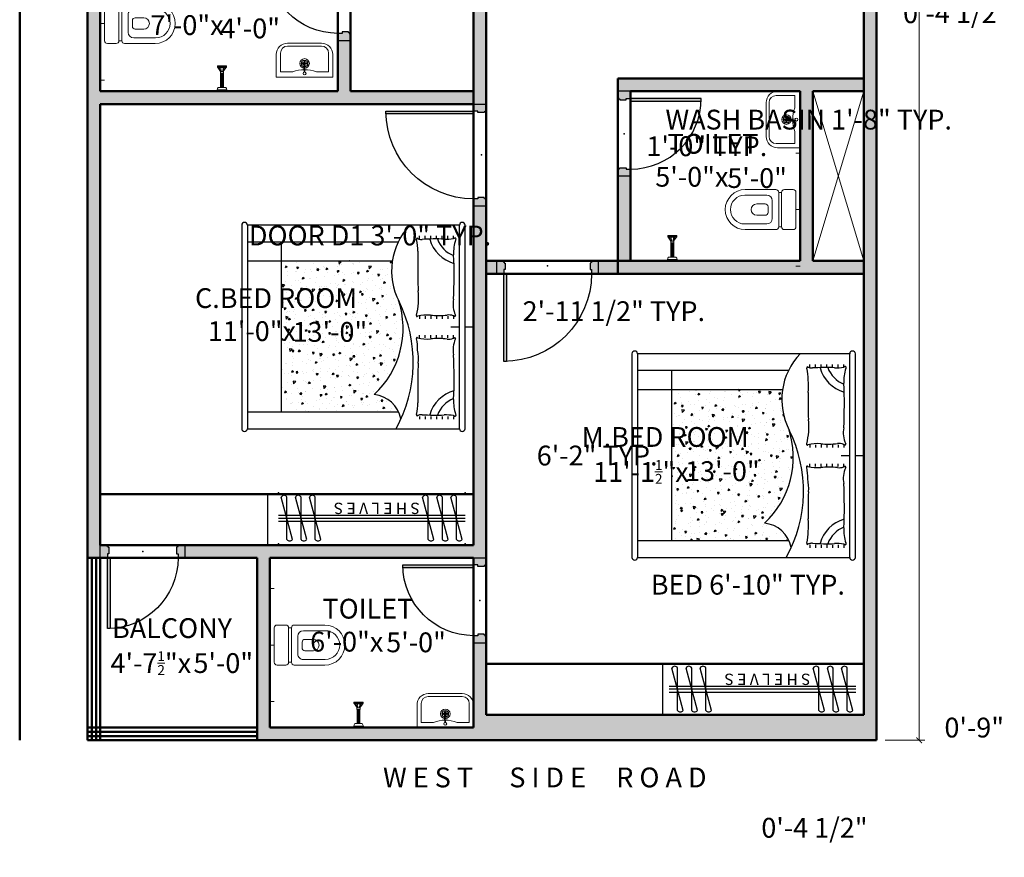
# Model space of a CAD drawing. Units: inches. Extents: x 4508 to 5907, y 877 to 1592.
# Tile 1 of 20: x 4571 to 4919, y 885 to 1182. Entities that reach past the tile are written whole.
import ezdxf

# ---------------------------------------------------------------- set-up
doc = ezdxf.new("R2010")
doc.units = ezdxf.units.IN
doc.layers.get('DEFPOINTS').update_dxf_attribs({"color": 8})
for name, color, linetype, lineweight in [('A-ANNO-DIMS', 2, 'Continuous', 18), ('A-ANNO-TEXT', 7, 'Continuous', 25), ('A-DOOR', 4, 'Continuous', 25), ('A-FLOR-CASE', 30, 'Continuous', 25), ('A-FLOR-FIXT', 8, 'Continuous', 18), ('A-FLOR-SHFT', 8, 'Continuous', 18), ('A-FURN', 24, 'Continuous', 18), ('A-WALL', 7, 'Continuous', 50), ('A-WALL-PATT', 8, 'Continuous', 13)]:
    doc.layers.add(name, color=color, linetype=linetype, lineweight=lineweight)
doc.layers.add('doors & windows', color=30, linetype='Continuous')
doc.layers.add('furniture', color=24, linetype='Continuous')
doc.styles.get("Standard").update_dxf_attribs({"font": 'arial.ttf'})
doc.dimstyles.new('details', dxfattribs={"dimtxt": 5, "dimasz": 2, "dimexe": 2, "dimexo": 3, "dimgap": 1, "dimtad": 0, "dimdec": 1, "dimzin": 0, "dimdsep": 46, "dimlunit": 4, "dimtxsty": 'Standard', "dimblk": 'ARCHTICK', "dimcen": 3, "dimclrd": 256, "dimclre": 256, "dimclrt": 256, "dimadec": 0, "dimazin": 0, "dimtfac": 0.5, "dimtdec": 1, "dimtofl": 0, "dimtmove": 0, "dimatfit": 3, "dimldrblk": 'CLOSEDBLANK', "dimfxl": 2, "dimtolj": 1, "dimtzin": 0, "dimlwd": -1, "dimlwe": -1, "dimarcsym": 0})
doc.dimstyles.new('text', dxfattribs={"dimtxt": 7, "dimasz": 0, "dimexe": 3, "dimexo": 3, "dimgap": 0, "dimtad": 1, "dimtih": 1, "dimtoh": 1, "dimzin": 3, "dimdsep": 46, "dimlunit": 4, "dimtxsty": 'Standard', "dimblk": 'CLOSEDBLANK', "dimcen": 3, "dimse1": 1, "dimse2": 1, "dimsd1": 1, "dimsd2": 1, "dimclrd": 256, "dimclre": 256, "dimclrt": 256, "dimadec": 0, "dimazin": 0, "dimtfac": 0.5, "dimtofl": 0, "dimtmove": 0, "dimatfit": 3, "dimfxl": 3, "dimtolj": 1, "dimtzin": 0, "dimlwd": -1, "dimlwe": -1, "dimarcsym": 0})

# ---------------------------------------------------------------- blocks, each defined once
blk = doc.blocks.new('*D34')
at = {"layer": 'DEFPOINTS', "color": 0, "transparency": 16777216}
for p in [(4683.74, 1178.32), (4683.74, 1175.99), (4599.74, 1170.14)]:
    blk.add_point(p, dxfattribs=at)
at = {"layer": 'A-ANNO-DIMS', "color": 0, "transparency": 16777216, "insert": (4630.42, 1185.46), "char_height": 7, "attachment_point": 5}
blk.add_mtext('\\A1;       TOILET\\P7\'-0"x', dxfattribs=at)
blk = doc.blocks.new('_ClosedBlank')
at = {"color": 0, "lineweight": -2}
for p, q in [((-1, 0.17), (0, 0)), ((-1, 0.17), (-1, -0.17)), ((0, 0), (-1, -0.17))]:
    blk.add_line(p, q, dxfattribs=at)
blk = doc.blocks.new('*D35')
at = {"layer": 'DEFPOINTS', "color": 0, "transparency": 16777216}
for p in [(4647.76, 1204.2), (4647.07, 1156.2), (4652.75, 1156.2)]:
    blk.add_point(p, dxfattribs=at)
at = {"layer": 'A-ANNO-DIMS', "color": 0, "transparency": 16777216, "insert": (4652.75, 1178.45), "char_height": 7, "attachment_point": 5}
blk.add_mtext('\\A1;4\'-0"', dxfattribs=at)
blk = doc.blocks.new('D2')
at = {"layer": 'doors & windows'}
h = blk.add_hatch(dxfattribs=at)
h.set_pattern_fill('DOTS', color=256, scale=2, angle=180, style=0)
h.set_pattern_definition([(180, (0, -4), (-0.0625, -0.125), [0, -0.125])])
h.paths.add_polyline_path([(2.5, 0), (3.5, 0), (3.5, 24.98, 0.010003), (2.5, 25)])
h = blk.add_hatch(dxfattribs=at)
h.set_pattern_fill('DOTS', color=256, scale=2, angle=180, style=0)
h.set_pattern_definition([(180, (0, 0), (-0.0625, -0.125), [0, -0.125])])
edge = h.paths.add_edge_path()
edge.add_line((27.5, 0), (27.5, -1.5))
edge.add_line((27.5, -1.5), (27, -1.5))
edge.add_line((27, -1.5), (27, -3.75))
edge.add_line((27, -3.75), (27.25, -3.75))
edge.add_arc((27.76, -3.74), 0.509, 181.0059, 268.9941)
edge.add_line((27.75, -4.25), (27.75, -4.5))
edge.add_line((27.75, -4.5), (30, -4.5))
edge.add_line((30, -4.5), (30, 0))
edge.add_line((30, 0), (27.5, 0))
edge = h.paths.add_edge_path()
edge.add_line((2.5, -1.5), (2.5, 0))
edge.add_line((2.5, 0), (0, 0))
edge.add_line((0, 0), (0, -4.5))
edge.add_line((0, -4.5), (2.25, -4.5))
edge.add_line((2.25, -4.5), (2.25, -4.25))
edge.add_arc((2.24, -3.74), 0.509, 271.0059, 358.9941)
edge.add_line((2.75, -3.75), (3, -3.75))
edge.add_line((3, -3.75), (3, -1.5))
edge.add_line((3, -1.5), (2.5, -1.5))
for p, q in [((0, 0), (0, -4.5)), ((30, 0), (30, -4.5))]:
    blk.add_line(p, q)
blk.add_lwpolyline([(3.5, 0), (3.5, 25), (2.5, 25), (2.5, 0)], close=True, dxfattribs=at)
for points in [[(3, -3.75), (3, -1.5), (2.5, -1.5), (2.5, 0), (0, 0)], [(27, -3.75), (27, -1.5), (27.5, -1.5), (27.5, 0), (30, 0)], [(0, -4.5), (2.25, -4.5)], [(30, -4.5), (27.75, -4.5)]]:
    blk.add_lwpolyline(points, dxfattribs=at)
for points in [[(2.25, -4.5), (2.25, -4.25, 0.403966), (2.75, -3.75), (3, -3.75)], [(27.75, -4.5), (27.75, -4.25, -0.403966), (27.25, -3.75), (27, -3.75)]]:
    blk.add_lwpolyline(points, format="xyb", dxfattribs=at)
at = {"layer": 'doors & windows', "ltscale": 6}
blk.add_arc((2.5, 0), 25, 0, 90, dxfattribs=at)
at = {"layer": 'doors & windows'}
blk.add_point((15, -2.25), dxfattribs=at)
blk = doc.blocks.new('commode')
for p, q in [((-7.09, 19.41), (-7.09, 8.61)), ((-5.09, 11.81), (-5.09, 19.57)), ((5.09, 11.81), (5.09, 19.57)), ((7.09, 19.41), (7.09, 8.61)), ((-2, 12.37), (-2, 15.37)), ((2, 12.37), (2, 15.37)), ((-1, 11.37), (1, 11.37)), ((-6.09, 7.61), (6.09, 7.61)), ((-6.09, 6.61), (-6.09, 7.61)), ((-3.15, 9.87), (3.15, 9.87)), ((6.09, 7.61), (6.09, 6.61)), ((-7.09, 2.5), (-7.09, 5.61)), ((-6.09, 6.61), (6.09, 6.61)), ((7.09, 2.5), (7.09, 5.61)), ((-20, 1.5), (-20, 0)), ((-6.09, 1.5), (6.09, 1.5)), ((0, 1.5), (0, 0)), ((20, 1.5), (20, 0))]:
    blk.add_line(p, q)
for centre, radius, start, end in [((0, 19.41), 7.09, 0, 180), ((0, 19.57), 5.09, 0, 180), ((0, 15.37), 2, 0, 180), ((-3.15, 11.81), 1.94, 180, 270), ((-1, 12.37), 1, 180, 270), ((1, 12.37), 1, 270, 0), ((3.15, 11.81), 1.94, 270, 0), ((-6.09, 8.61), 1, 180, 270), ((6.09, 8.61), 1, 270, 0), ((-6.09, 5.61), 1, 90, 180), ((6.09, 5.61), 1, 0, 90), ((-6.09, 2.5), 1, 180, 270), ((6.09, 2.5), 1, 270, 0)]:
    blk.add_arc(centre, radius, start, end)
blk = doc.blocks.new('wash basin 1')
for p, q in [((-8.5, 8.5), (-1.85, 8.5)), ((0, 10), (-8, 10)), ((-1.85, 8.5), (-1.85, 4.19)), ((0, 10), (0, -10)), ((-12, 6), (-12, -6)), ((-11, 6), (-11, -6)), ((-1.85, -8.5), (-1.85, -4.19)), ((-8.5, -8.5), (-1.85, -8.5)), ((0, -10), (-8, -10))]:
    blk.add_line(p, q)
blk.add_lwpolyline([(-1.83, 0.11), (-5.25, 0.25), (-5.23, -0.38), (-1.8, -0.19)])
for centre, radius in [((-4.87, 0), 1.68), ((-4.87, 0), 1.18), ((-5.63, 0), 0.25), ((-4.87, 0.75), 0.25), ((-4.87, 0), 0.25), ((-4.19, 0), 0.25), ((-1.34, 0), 0.5), ((-4.87, -0.72), 0.25)]:
    blk.add_circle(centre, radius)
for centre, radius, start, end in [((-8, 6), 4, 90, 180), ((-8.5, 6), 2.5, 90, 180), ((8.89, 0), 11.53, 158.7059, 201.2941), ((-8, -6), 4, 180, 270), ((-8.5, -6), 2.5, 180, 270)]:
    blk.add_arc(centre, radius, start, end)
blk = doc.blocks.new('tap & shower')
for p, q in [((1.71, 0), (-1.71, 0)), ((-1.71, 0), (-1.71, -0.5)), ((1.71, 0), (1.71, -0.5)), ((1.71, -0.5), (-1.71, -0.5)), ((1.31, -1.4), (-1.31, -1.4)), ((-0.5, -6.44), (-0.5, -1.4)), ((-0.42, -6.44), (-0.42, -1.4)), ((-0.32, -0.5), (0.32, -0.5)), ((-0.3, -6.44), (-0.3, -1.4)), ((-0.14, -6.44), (-0.14, -1.4)), ((0.14, -6.44), (0.14, -1.4)), ((0.3, -6.44), (0.3, -1.4)), ((0.42, -6.44), (0.42, -1.4)), ((0.5, -6.44), (0.5, -1.4)), ((-0.56, -6.44), (0.56, -6.44)), ((-0.56, -6.98), (-0.56, -6.44)), ((0.56, -6.98), (0.56, -6.44)), ((-1.62, -8.87), (-1.62, -8.6)), ((-1.48, -8.46), (-0.47, -6.98)), ((-1.48, -8.46), (1.48, -8.46)), ((-1.48, -9), (-1.48, -8.46)), ((-1.48, -9), (1.48, -9)), ((-1.43, -9), (-1.43, -8.46)), ((-1.37, -9), (-1.37, -8.46)), ((-1.32, -9), (-1.32, -8.46)), ((-1.27, -9), (-1.27, -8.46)), ((-1.21, -9), (-1.21, -8.46)), ((-1.16, -9), (-1.16, -8.46)), ((-1.1, -9), (-1.1, -8.46)), ((-1.05, -9), (-1.05, -8.46)), ((-1, -9), (-1, -8.46)), ((-0.41, -6.98), (-0.94, -8.46)), ((-0.94, -9), (-0.94, -8.46)), ((-0.89, -9), (-0.89, -8.46)), ((-0.84, -9), (-0.84, -8.46)), ((-0.78, -9), (-0.78, -8.46)), ((-0.73, -9), (-0.73, -8.46)), ((-0.67, -9), (-0.67, -8.46)), ((-0.62, -9), (-0.62, -8.46)), ((-0.57, -9), (-0.57, -8.46)), ((-0.56, -6.98), (0.56, -6.98)), ((-0.51, -9), (-0.51, -8.46)), ((-0.46, -9), (-0.46, -8.46)), ((-0.29, -6.98), (-0.4, -8.46)), ((-0.4, -9), (-0.4, -8.46)), ((-0.35, -9), (-0.35, -8.46)), ((-0.3, -9), (-0.3, -8.46)), ((-0.24, -9), (-0.24, -8.46)), ((-0.19, -9), (-0.19, -8.46)), ((-0.13, -9), (-0.13, -8.46)), ((-0.08, -9), (-0.08, -8.46)), ((-0.03, -9), (-0.03, -8.46)), ((0.03, -9), (0.03, -8.46)), ((0.08, -9), (0.08, -8.46)), ((0.13, -9), (0.13, -8.46)), ((0.19, -9), (0.19, -8.46)), ((0.24, -9), (0.24, -8.46)), ((0.29, -6.98), (0.4, -8.46)), ((0.3, -9), (0.3, -8.46)), ((0.35, -9), (0.35, -8.46)), ((0.4, -9), (0.4, -8.46)), ((0.41, -6.98), (0.94, -8.46)), ((0.46, -9), (0.46, -8.46)), ((1.48, -8.46), (0.47, -6.98)), ((0.51, -9), (0.51, -8.46)), ((0.57, -9), (0.57, -8.46)), ((0.62, -9), (0.62, -8.46)), ((0.67, -9), (0.67, -8.46)), ((0.73, -9), (0.73, -8.46)), ((0.78, -9), (0.78, -8.46)), ((0.84, -9), (0.84, -8.46)), ((0.89, -9), (0.89, -8.46)), ((0.94, -9), (0.94, -8.46)), ((1, -9), (1, -8.46)), ((1.05, -9), (1.05, -8.46)), ((1.1, -9), (1.1, -8.46)), ((1.16, -9), (1.16, -8.46)), ((1.21, -9), (1.21, -8.46)), ((1.27, -9), (1.27, -8.46)), ((1.32, -9), (1.32, -8.46)), ((1.37, -9), (1.37, -8.46)), ((1.43, -9), (1.43, -8.46)), ((1.48, -9), (1.48, -8.46)), ((1.62, -8.87), (1.62, -8.6))]:
    blk.add_line(p, q)
for centre, radius, start, end in [((-0.02, -0.29), 1.7, 187.1825, 220.9028), ((0.02, -0.29), 1.7, 319.0972, 352.8175), ((-1.48, -8.6), 0.135, 90, 180), ((-1.48, -8.87), 0.135, 180, 270), ((1.48, -8.6), 0.135, 0, 90), ((1.48, -8.87), 0.135, 270, 0)]:
    blk.add_arc(centre, radius, start, end)
blk = doc.blocks.new('D1')
at = {"layer": 'doors & windows'}
h = blk.add_hatch(dxfattribs=at)
h.set_pattern_fill('DOTS', color=256, scale=2, angle=180, style=0)
h.set_pattern_definition([(180, (-2e-12, -4), (-0.0625, -0.125), [0, -0.125])])
h.paths.add_polyline_path([(2.5, 0), (3.5, 0), (3.5, 30.98, 0.008066), (2.5, 31)])
h = blk.add_hatch(dxfattribs=at)
h.set_pattern_fill('DOTS', color=256, scale=2, angle=180, style=0)
h.set_pattern_definition([(180, (0, -0.5), (-0.0625, -0.125), [0, -0.125])])
h.paths.add_polyline_path([(0, -4.5), (2.25, -4.5), (2.25, -4.25, 0.403966), (2.75, -3.75), (3, -3.75), (3, -1.5), (2.5, -1.5), (2.5, 0), (0, 0)])
h.paths.add_polyline_path([(36, -4.5), (36, 0), (33.5, 0), (33.5, -1.5), (33, -1.5), (33, -3.75), (33.25, -3.75, 0.403966), (33.75, -4.25), (33.75, -4.5)])
for p, q in [((0, 0), (0, -4.5)), ((36, 0), (36, -4.5))]:
    blk.add_line(p, q)
blk.add_lwpolyline([(3.5, 0), (3.5, 31), (2.5, 31), (2.5, 0)], close=True, dxfattribs=at)
for points in [[(3, -3.75), (3, -1.5), (2.5, -1.5), (2.5, 0), (0, 0)], [(33, -3.75), (33, -1.5), (33.5, -1.5), (33.5, 0), (36, 0)], [(0, -4.5), (2.25, -4.5)], [(36, -4.5), (33.75, -4.5)]]:
    blk.add_lwpolyline(points, dxfattribs=at)
for points in [[(2.25, -4.5), (2.25, -4.25, 0.403966), (2.75, -3.75), (3, -3.75)], [(33.75, -4.5), (33.75, -4.25, -0.403966), (33.25, -3.75), (33, -3.75)]]:
    blk.add_lwpolyline(points, format="xyb", dxfattribs=at)
at = {"layer": 'doors & windows', "ltscale": 6}
blk.add_arc((2.5, 0), 31, 0, 90, dxfattribs=at)
at = {"layer": 'doors & windows'}
blk.add_point((18, -2.75), dxfattribs=at)
blk = doc.blocks.new('*D36')
at = {"layer": 'DEFPOINTS', "color": 0, "transparency": 16777216}
for p in [(4731.74, 961.2), (4731.74, 957.95), (4659.74, 955.96)]:
    blk.add_point(p, dxfattribs=at)
at = {"layer": 'A-ANNO-DIMS', "color": 0, "transparency": 16777216, "insert": (4686.89, 967.42), "char_height": 7, "attachment_point": 5}
blk.add_mtext('\\A1;       TOILET\\P6\'-0"x', dxfattribs=at)
blk = doc.blocks.new('*D37')
at = {"layer": 'DEFPOINTS', "color": 0, "transparency": 16777216}
for p in [(4695.74, 991.2), (4701.57, 931.2), (4711.4, 931.2)]:
    blk.add_point(p, dxfattribs=at)
at = {"layer": 'A-ANNO-DIMS', "color": 0, "transparency": 16777216, "insert": (4711.4, 961.35), "char_height": 7, "attachment_point": 5}
blk.add_mtext('\\A1;5\'-0"', dxfattribs=at)
blk = doc.blocks.new('*D38')
at = {"layer": 'DEFPOINTS', "color": 0, "transparency": 16777216}
for p in [(4599.74, 955.46), (4655.24, 953.31), (4655.24, 949.85)]:
    blk.add_point(p, dxfattribs=at)
at = {"layer": 'A-ANNO-DIMS', "color": 0, "transparency": 16777216, "insert": (4617.62, 959.84), "char_height": 7, "attachment_point": 5}
blk.add_mtext('\\A1;       BALCONY\\P4\'-7{\\H0.5x;\\S1/2;}"x', dxfattribs=at)
blk = doc.blocks.new('*D39')
at = {"layer": 'DEFPOINTS', "color": 0, "transparency": 16777216}
for p in [(4634.75, 991.2), (4634.71, 931.2), (4643.23, 931.2)]:
    blk.add_point(p, dxfattribs=at)
at = {"layer": 'A-ANNO-DIMS', "color": 0, "transparency": 16777216, "insert": (4643.23, 954.02), "char_height": 7, "attachment_point": 5}
blk.add_mtext('\\A1;5\'-0"', dxfattribs=at)
blk = doc.blocks.new('hangers')
at = {"layer": 'furniture'}
for p, q in [((1, 7.5), (5, -7.5)), ((3, 7.5), (3, -7.5)), ((6, 7.5), (10, -7.5)), ((8, 7.5), (8, -7.5)), ((11, 7.5), (15, -7.5)), ((13, 7.5), (13, -7.5)), ((51, 7.5), (55, -7.5)), ((53, 7.5), (53, -7.5)), ((56, 7.5), (60, -7.5)), ((58, 7.5), (58, -7.5)), ((61, 7.5), (65, -7.5)), ((63, 7.5), (63, -7.5)), ((66, 1), (0, 1)), ((0, 0), (66, 0)), ((0, -1), (66, -1))]:
    blk.add_line(p, q, dxfattribs=at)
for centre, radius, start, end in [((2, 6.62), 1.33, 41.2884, 138.7116), ((7, 6.62), 1.33, 41.2884, 138.7116), ((12, 6.62), 1.33, 41.2884, 138.7116), ((52, 6.62), 1.33, 41.2884, 138.7116), ((57, 6.62), 1.33, 41.2884, 138.7116), ((62, 6.62), 1.33, 41.2884, 138.7116), ((4, -7.08), 1.08, 202.5549, 337.4451), ((9, -7.08), 1.08, 202.5549, 337.4451), ((14, -7.08), 1.08, 202.5549, 337.4451), ((54, -7.08), 1.08, 202.5549, 337.4451), ((59, -7.08), 1.08, 202.5549, 337.4451), ((64, -7.08), 1.08, 202.5549, 337.4451)]:
    blk.add_arc(centre, radius, start, end, dxfattribs=at)
for p in [(0, 9), (66, 9), (0, -9), (66, -9)]:
    blk.add_point(p, dxfattribs=at)
blk.add_text('S H E L V E S', height=4, dxfattribs=at).set_placement((16, -5.52))
blk = doc.blocks.new('*D40')
at = {"layer": 'DEFPOINTS', "color": 0, "transparency": 16777216}
for p in [(4672, 1151.7), (4664.67, 995.7), (4680.94, 995.7)]:
    blk.add_point(p, dxfattribs=at)
at = {"layer": 'A-ANNO-DIMS', "color": 0, "transparency": 16777216, "insert": (4680.94, 1071.13), "char_height": 7, "attachment_point": 5}
blk.add_mtext('\\A1;13\'-0"', dxfattribs=at)
blk = doc.blocks.new('*D41')
at = {"layer": 'DEFPOINTS', "color": 0, "transparency": 16777216}
for p in [(4731.74, 1075.98), (4599.74, 1073.7), (4731.74, 1067.77)]:
    blk.add_point(p, dxfattribs=at)
at = {"layer": 'A-ANNO-DIMS', "color": 0, "transparency": 16777216, "insert": (4653.36, 1077.24), "char_height": 7, "attachment_point": 5}
blk.add_mtext('\\A1;        C.BED ROOM\\P11\'-0"x', dxfattribs=at)
blk = doc.blocks.new('bed')
at = {"layer": 'furniture'}
h = blk.add_hatch(dxfattribs=at)
h.set_pattern_fill('AR-CONC', color=256, angle=-90, style=0)
h.set_pattern_definition([(320, (0, 2.38), (-0.6275, -7.1726), [0.75, -8.25]), (265, (0, 2.38), (7.5219, 1.3875), [0.6, -6.6]), (10.451, (-0.052, 1.782), (6.8944, -5.7851), [0.6374, -7.0114]), (316.184, (2, 2.38), (-1.6552, -10.6724), [1.125, -12.375]), (6.636, (1.862, 1.491), (9.7412, -9.3466), [0.9561, -10.5171]), (261.184, (2, 2.38), (9.7412, -9.3466), [0.9, -9.9]), (291, (1.5, 1.38), (-4.0262, -5.96907), [0.75, -8.25]), (236, (1.5, 1.38), (7.2515, -2.43315), [0.6, -6.6]), (341.451, (1.1645, 0.8826), (3.2253, -8.4022), [0.6374, -7.0114]), (307.5, (0, 2.38), (3.32894, -0.1216), [0, -6.52, 0, -6.7, 0, -6.625]), (277.5, (0, 2.38), (3.94412, -2.6307), [0, -3.82, 0, -6.37, 0, -2.525]), (237.5, (0, 4.61), (-0.22555, -5.33822), [0, -2.5, 0, -7.8, 0, -10.35]), (227.5, (0, 5.61), (1.00105, -5.83186), [0, -3.25, 0, -5.18, 0, -7.35])])
h.paths.add_polyline_path([(30.01, -68), (30.01, -26.5, 0.263043), (23.9, -35.15, 0.293424), (-9.18, -26.47, -0.156683), (-23.39, -28.72), (-23.39, -68)])
for p, q in [((0, -3), (0, 0)), ((36.01, -3), (-36.01, -3)), ((-36.01, -5), (-36.01, -80)), ((36.01, -5), (-36.01, -5)), ((0, -8), (0, -5)), ((36.01, -80), (36.01, -5)), ((-31.24, -7.07), (-32.24, -7.07)), ((-31.24, -9.07), (-32.24, -9.07)), ((-3.81, -7.07), (-2.81, -7.07)), ((-3.81, -9.07), (-2.81, -9.07)), ((3.89, -7.07), (2.89, -7.07)), ((3.89, -9.07), (2.89, -9.07)), ((31.63, -7.07), (32.63, -7.07)), ((31.63, -9.07), (32.63, -9.07)), ((-31.24, -11.07), (-32.24, -11.07)), ((-31.24, -13.07), (-32.24, -13.07)), ((-3.81, -11.07), (-2.81, -11.07)), ((-3.81, -13.07), (-2.81, -13.07)), ((3.89, -11.07), (2.89, -11.07)), ((3.89, -13.07), (2.89, -13.07)), ((31.63, -11.07), (32.63, -11.07)), ((31.63, -13.07), (32.63, -13.07)), ((-31.24, -15.07), (-32.24, -15.07)), ((-31.24, -17.07), (-32.24, -17.07)), ((-3.81, -15.07), (-2.81, -15.07)), ((-3.81, -17.07), (-2.81, -17.07)), ((3.89, -15.07), (2.89, -15.07)), ((3.89, -17.07), (2.89, -17.07)), ((31.63, -15.07), (32.63, -15.07)), ((31.63, -17.07), (32.63, -17.07)), ((-31.24, -19.07), (-32.24, -19.07)), ((-3.81, -19.07), (-2.81, -19.07)), ((3.89, -19.07), (2.89, -19.07)), ((31.63, -19.07), (32.63, -19.07)), ((-36.01, -80), (36.01, -80)), ((-36.01, -82), (36.01, -82))]:
    blk.add_line(p, q, dxfattribs=at)
at = {"layer": 'furniture', "ltscale": 5}
blk.add_line((-30.01, -26.66), (-30.01, -80), dxfattribs=at)
at = {"layer": 'furniture', "ltscale": 7}
blk.add_line((30.01, -80), (30.01, -26.5), dxfattribs=at)
at = {"layer": 'furniture', "ltscale": 0.3}
for p, q in [((-23.39, -80), (-23.39, -28.72)), ((-30.01, -68), (30.01, -68))]:
    blk.add_line(p, q, dxfattribs=at)
at = {"layer": 'furniture'}
for centre, radius, start, end in [((-35.95, -4), 1, 93.3831, 266.6169), ((35.95, -4), 1, 273.3831, 86.6169), ((-31.1, -6.57), 0.382, 35.8976, 208.6272), ((-44.44, -13.85), 14.82, 27.1629, 28.6272), ((-34.45, -3.51), 12.47, 286.0319, 344.1205), ((-26.35, 6.68), 13.76, 251.1782, 273.3982), ((-18.02, -163.6), 156.72, 87.0032, 92.7497), ((-8.03, 2.03), 9.29, 258.896, 294.7184), ((-4.03, -6.67), 0.282, 335.7259, 114.303), ((3.22, -9.94), 7.68, 155.7259, 159.0146), ((4.11, -6.67), 0.282, 65.697, 204.2741), ((-3.14, -9.94), 7.68, 20.9854, 24.2741), ((8.12, 2.03), 9.29, 245.2816, 281.104), ((18.1, -163.6), 156.72, 87.2503, 92.9968), ((34.54, -3.51), 12.47, 195.8795, 253.9681), ((26.43, 6.68), 13.76, 266.6018, 288.8218), ((31.18, -6.57), 0.382, 331.3728, 144.1024), ((44.53, -13.85), 14.82, 151.3728, 152.8371), ((-46.76, -9.65), 15.72, 357.4804, 9.3956), ((54.88, -13.16), 85.99, 178.1209, 183.3613), ((-34.45, -3.51), 9.85, 289.8695, 338.9843), ((0.25, -8.8), 4.49, 159.0146, 186.273), ((-32.82, -12.44), 28.78, 354.3784, 6.273), ((-0.17, -8.8), 4.49, 353.727, 20.9854), ((32.9, -12.44), 28.78, 173.727, 185.6216), ((34.54, -3.51), 9.85, 201.0157, 250.1305), ((-54.8, -13.16), 85.99, 356.6387, 1.8791), ((46.84, -9.65), 15.72, 170.6044, 182.5196), ((-28.62, 31.03), 42.31, 266.4836, 266.6487), ((28.7, 31.03), 42.31, 273.3513, 273.5164), ((12.28, -16.11), 16.48, 177.0317, 192.8678), ((-12.19, -16.11), 16.48, 347.1322, 2.9683), ((-31.05, -19.91), 0.291, 147.6219, 311.9343), ((-33.2, -18.55), 2.25, 327.6219, 339.2246), ((-34.13, -18.41), 3.18, 342.7809, 3.755), ((-24.4, -58.01), 38.42, 93.5164, 99.6766), ((-24.52, -56.06), 36.48, 86.4836, 93.5164), ((-18.49, 70.49), 90.23, 267.5921, 273.6329), ((-10.31, -44.95), 25.52, 75.952, 95.5452), ((-3.95, -19.99), 0.265, 231.9005, 52.8902), ((4.03, -19.99), 0.265, 127.1098, 308.0995), ((7.57, -34.68), 14.87, 87.3976, 103.1191), ((11.44, -34.81), 15.32, 84.694, 102.0355), ((18.57, 70.49), 90.23, 266.3671, 272.4079), ((24.6, -56.06), 36.48, 86.4836, 93.5164), ((24.48, -58.01), 38.42, 80.3234, 86.4836), ((31.13, -19.91), 0.291, 228.0657, 32.3781), ((34.21, -18.41), 3.18, 176.245, 197.2191), ((33.28, -18.55), 2.25, 200.7754, 212.3781), ((-19.79, -5.47), 23.53, 226.4061, 297.4441), ((12.51, -69.71), 48.38, 60.9345, 116.3227), ((0.6, -56.57), 31.65, 42.5874, 108.5034), ((34.61, -36.23), 10.76, 101.1719, 174.259), ((-35.95, -81), 1, 93.3831, 266.6169), ((35.95, -81), 1, 273.3831, 86.6169)]:
    blk.add_arc(centre, radius, start, end, dxfattribs=at)
blk = doc.blocks.new('*D42')
at = {"layer": 'DEFPOINTS', "color": 0, "transparency": 16777216}
for p in [(4850.06, 1125.98), (4850.06, 1122.35), (4790.06, 1116.29)]:
    blk.add_point(p, dxfattribs=at)
at = {"layer": 'A-ANNO-DIMS', "color": 0, "transparency": 16777216, "insert": (4808.93, 1131.82), "char_height": 7, "attachment_point": 5}
blk.add_mtext('\\A1;       TOILET\\P5\'-0"x', dxfattribs=at)
blk = doc.blocks.new('*D43')
at = {"layer": 'DEFPOINTS', "color": 0, "transparency": 16777216}
for p in [(4818.74, 1155.98), (4818.74, 1095.98), (4832, 1095.98)]:
    blk.add_point(p, dxfattribs=at)
at = {"layer": 'A-ANNO-DIMS', "color": 0, "transparency": 16777216, "insert": (4832, 1125.53), "char_height": 7, "attachment_point": 5}
blk.add_mtext('\\A1;5\'-0"', dxfattribs=at)
blk = doc.blocks.new('*D44')
at = {"layer": 'DEFPOINTS', "color": 0, "transparency": 16777216}
for p in [(4808.19, 1091.7), (4802.99, 935.7), (4819.72, 935.7)]:
    blk.add_point(p, dxfattribs=at)
at = {"layer": 'A-ANNO-DIMS', "color": 0, "transparency": 16777216, "insert": (4819.72, 1021.89), "char_height": 7, "attachment_point": 5}
blk.add_mtext('\\A1;13\'-0"', dxfattribs=at)
blk = doc.blocks.new('*D45')
at = {"layer": 'DEFPOINTS', "color": 0, "transparency": 16777216}
for p in [(4869.74, 1017.45), (4736.24, 1014.28), (4869.74, 1014.28)]:
    blk.add_point(p, dxfattribs=at)
at = {"layer": 'A-ANNO-DIMS', "color": 0, "transparency": 16777216, "insert": (4790.92, 1027.44), "char_height": 7, "attachment_point": 5}
blk.add_mtext('\\A1;        M.BED ROOM\\P11\'-1{\\H0.5x;\\S1/2;}"x', dxfattribs=at)
blk = doc.blocks.new('*D47')
at = {"layer": 'DEFPOINTS', "color": 0, "transparency": 16777216}
for p in [(4826.39, 1328.7), (4829.43, 1328.7), (4817.29, 1160.7)]:
    blk.add_point(p, dxfattribs=at)
at = {"layer": 'A-ANNO-DIMS', "color": 0, "transparency": 16777216, "insert": (4826.39, 1234.84), "char_height": 7, "attachment_point": 5}
blk.add_mtext('\\A1;14\'-0"', dxfattribs=at)
blk = doc.blocks.new('_ArchTick')
at = {"color": 0, "linetype": 'ByBlock', "const_width": 0.15}
blk.add_lwpolyline([(-0.5, -0.5), (0.5, 0.5)], dxfattribs=at)
blk = doc.blocks.new('*D52')
at = {"layer": 'A-ANNO-DIMS', "color": 0, "transparency": 16777216}
for p, q in [((4877.24, 1574.7), (4891.29, 1574.7)), ((4889.29, 1574.7), (4889.29, 1255.95)), ((4889.29, 926.7), (4889.29, 1245.46)), ((4877.24, 926.7), (4891.29, 926.7))]:
    blk.add_line(p, q, dxfattribs=at)
at = {"layer": 'DEFPOINTS', "color": 0, "transparency": 16777216}
for p in [(4874.24, 1574.7), (4874.24, 926.7), (4889.29, 926.7)]:
    blk.add_point(p, dxfattribs=at)
at = {"layer": 'A-ANNO-DIMS', "color": 0, "transparency": 16777216, "xscale": 2, "yscale": 2, "zscale": 2}
for p, rotation in [((4889.29, 1574.7), 90), ((4889.29, 926.7), 270)]:
    blk.add_blockref('_ArchTick', p, dxfattribs=dict(at, rotation=rotation))
at = {"layer": 'A-ANNO-DIMS', "color": 0, "transparency": 16777216, "insert": (4889.29, 1250.7), "char_height": 5, "attachment_point": 5, "rotation": 90}
blk.add_mtext("\\A1;54'", dxfattribs=at)
blk = doc.blocks.new('*D144')
at = {"layer": 'DEFPOINTS', "color": 0, "transparency": 16777216}
for p in [(4775.93, 1101.6), (4739.93, 1096.2), (4775.93, 1096.2)]:
    blk.add_point(p, dxfattribs=at)
at = {"layer": 'A-ANNO-DIMS', "transparency": 16777216, "insert": (4695.14, 1105.23), "char_height": 7, "attachment_point": 5}
blk.add_mtext('\\A1;DOOR D1 3\'-0" TYP.', dxfattribs=at)
blk = doc.blocks.new('*D145')
at = {"layer": 'DEFPOINTS', "color": 0, "transparency": 16777216}
for p in [(4775.93, 1096.2), (4775.93, 1060.7), (4781.33, 1060.7)]:
    blk.add_point(p, dxfattribs=at)
at = {"layer": 'A-ANNO-DIMS', "transparency": 16777216, "insert": (4781.33, 1078.45), "char_height": 7, "attachment_point": 5}
blk.add_mtext('\\A1;2\'-11 1/2" TYP.', dxfattribs=at)
blk = doc.blocks.new('*D152')
at = {"layer": 'DEFPOINTS', "color": 0, "transparency": 16777216}
for p in [(4787.74, 990.46), (4869.74, 990.46), (4869.74, 978.16)]:
    blk.add_point(p, dxfattribs=at)
at = {"layer": 'A-ANNO-DIMS', "transparency": 16777216, "insert": (4828.74, 981.73), "char_height": 7, "attachment_point": 5}
blk.add_mtext('\\A1;BED 6\'-10" TYP.', dxfattribs=at)
blk = doc.blocks.new('*D153')
at = {"layer": 'DEFPOINTS', "color": 0, "transparency": 16777216}
for p in [(4787.74, 1064.37), (4775.44, 990.46), (4787.74, 990.46)]:
    blk.add_point(p, dxfattribs=at)
at = {"layer": 'A-ANNO-DIMS', "transparency": 16777216, "insert": (4775.44, 1027.41), "char_height": 7, "attachment_point": 5}
blk.add_mtext('\\A1;6\'-2" TYP.', dxfattribs=at)
blk = doc.blocks.new('*D158')
at = {"layer": 'DEFPOINTS', "color": 0, "transparency": 16777216}
for p in [(4847.24, 1156.2), (4850.24, 1156.2), (4847.24, 1136.2)]:
    blk.add_point(p, dxfattribs=at)
at = {"layer": 'A-ANNO-DIMS', "transparency": 16777216, "insert": (4850.24, 1146.2), "char_height": 7, "attachment_point": 5}
blk.add_mtext('\\A1;WASH BASIN 1\'-8" TYP.', dxfattribs=at)
blk = doc.blocks.new('*D159')
at = {"layer": 'DEFPOINTS', "color": 0, "transparency": 16777216}
for p in [(4835.24, 1136.2), (4847.24, 1136.2), (4847.24, 1133.2)]:
    blk.add_point(p, dxfattribs=at)
at = {"layer": 'A-ANNO-DIMS', "transparency": 16777216, "insert": (4814.23, 1136.78), "char_height": 7, "attachment_point": 5}
blk.add_mtext('\\A1;1\'-0" TYP.', dxfattribs=at)
blk = doc.blocks.new('*D182')
at = {"layer": 'DEFPOINTS', "color": 0, "transparency": 16777216}
for p in [(4869.737064, 935.703772), (4908.787064, 935.703772), (4874.237064, 926.703772)]:
    blk.add_point(p, dxfattribs=at)
at = {"layer": 'A-ANNO-DIMS', "transparency": 16777216, "insert": (4908.787064, 931.203772), "char_height": 7, "attachment_point": 5}
blk.add_mtext('\\A1;0\'-9"', dxfattribs=at)
blk = doc.blocks.new('*D183')
at = {"layer": 'DEFPOINTS', "color": 0, "transparency": 16777216}
for p in [(4869.74, 935.7), (4874.24, 926.7), (4874.24, 892.15)]:
    blk.add_point(p, dxfattribs=at)
at = {"layer": 'A-ANNO-DIMS', "transparency": 16777216, "insert": (4852.28, 895.77), "char_height": 7, "attachment_point": 5}
blk.add_mtext('\\A1;0\'-4 1/2"', dxfattribs=at)
blk = doc.blocks.new('*D187')
at = {"layer": 'DEFPOINTS', "color": 0, "transparency": 16777216}
for p in [(4884.94, 1184.7), (4923.99, 1184.7), (4923.99, 1180.2)]:
    blk.add_point(p, dxfattribs=at)
at = {"layer": 'A-ANNO-DIMS', "transparency": 16777216, "insert": (4902.4, 1183.82), "char_height": 7, "attachment_point": 5}
blk.add_mtext('\\A1;0\'-4 1/2"', dxfattribs=at)

msp = doc.modelspace()

# ---------------------------------------------------------------- hatches: boundary and pattern name
at = {"layer": 'A-WALL-PATT'}
h = msp.add_hatch(color=256, dxfattribs=at)
h.dxf.hatch_style = 1
h.paths.add_polyline_path([(4874.237, 926.704), (4874.237, 1481.704), (4869.737, 1481.704), (4869.737, 1385.704), (4787.237, 1385.704), (4787.237, 1395.704), (4782.737, 1395.704), (4782.737, 1385.704), (4782.737, 1381.204), (4787.237, 1381.204), (4847.237, 1381.204), (4869.737, 1381.204), (4869.737, 1333.204), (4847.237, 1333.204), (4787.237, 1333.204), (4787.237, 1345.204), (4782.737, 1345.204), (4782.737, 1328.704), (4869.737, 1328.704), (4869.737, 935.704), (4736.237, 935.704), (4736.237, 961.204), (4731.737, 961.204), (4731.737, 931.204), (4711.737, 931.204), (4659.737, 931.204), (4659.737, 991.204), (4731.737, 991.204), (4736.237, 991.204), (4736.237, 1115.704), (4731.737, 1115.704), (4731.737, 995.704), (4629.737, 995.704), (4629.737, 991.204), (4655.237, 991.204), (4655.237, 926.704)])
h.paths.add_polyline_path([(4599.737, 1151.704), (4731.737, 1151.704), (4731.737, 1156.204), (4688.237, 1156.204), (4688.237, 1174.204), (4683.737, 1174.204), (4683.737, 1156.204), (4599.737, 1156.204), (4599.737, 1204.204), (4683.737, 1204.204), (4688.237, 1204.204), (4688.237, 1208.704), (4599.737, 1208.704), (4599.737, 1328.704), (4731.737, 1328.704), (4731.737, 1321.757), (4736.237, 1321.757), (4736.237, 1333.204), (4599.737, 1333.204), (4599.737, 1481.704), (4606.251, 1481.704), (4606.251, 1490.704), (4595.237, 1490.704), (4595.237, 991.204), (4599.737, 991.204), (4599.737, 995.704)])
h.paths.add_polyline_path([(4736.237, 1285.757), (4731.737, 1285.757), (4731.737, 1151.704), (4736.237, 1151.704)], flags=17)
h = msp.add_hatch(color=256, dxfattribs=at)
h.dxf.hatch_style = 1
h.paths.add_polyline_path([(4869.737, 1096.204), (4851.737, 1096.204), (4851.737, 1156.204), (4869.737, 1156.204), (4869.737, 1160.704), (4782.737, 1160.704), (4782.737, 1156.204), (4787.237, 1156.204), (4847.237, 1156.204), (4847.237, 1136.204), (4847.237, 1096.204), (4787.237, 1096.204), (4787.237, 1126.204), (4782.737, 1126.204), (4782.737, 1091.704), (4869.737, 1091.704)])
h = msp.add_hatch(color=256, dxfattribs=at)
h.dxf.hatch_style = 1
h.paths.add_polyline_path([(4782.737, 1096.204), (4775.933, 1096.204), (4775.933, 1091.704), (4782.737, 1091.704)])
h.paths.add_polyline_path([(4739.933, 1096.204), (4736.237, 1096.204), (4736.237, 1091.704), (4739.933, 1091.704)])

# ---------------------------------------------------------------- linework, layer by layer
at = {"layer": 'A-FLOR-CASE'}
for p, q in [((4658.839, 1013.704), (4658.839, 995.704)), ((4798.592, 953.656), (4798.592, 935.656))]:
    msp.add_line(p, q, dxfattribs=at)
at = {"layer": 'A-FLOR-SHFT'}
for p, q in [((4851.737, 1156.204), (4869.737, 1096.204)), ((4851.737, 1096.204), (4869.737, 1156.204))]:
    msp.add_line(p, q, dxfattribs=at)
at = {"layer": 'A-WALL'}
for p, q in [((4571.237, 1574.704), (4571.237, 926.704)), ((4595.237, 1574.704), (4595.237, 926.704)), ((4874.237, 1574.704), (4874.237, 926.704)), ((4736.237, 1333.204), (4736.237, 935.704)), ((4731.737, 1328.704), (4731.737, 995.704)), ((4869.737, 1328.704), (4869.737, 935.704)), ((4688.237, 1208.704), (4688.237, 1156.204)), ((4599.737, 1204.204), (4599.737, 1156.204)), ((4683.737, 1204.204), (4683.737, 1156.204)), ((4782.737, 1160.704), (4869.737, 1160.704)), ((4782.737, 1160.704), (4782.737, 1091.704)), ((4599.737, 1156.204), (4683.737, 1156.204)), ((4688.237, 1156.204), (4731.737, 1156.204)), ((4787.237, 1156.204), (4847.237, 1156.204)), ((4787.237, 1156.204), (4787.237, 1096.204)), ((4847.237, 1156.204), (4847.237, 1096.204)), ((4851.737, 1156.204), (4851.737, 1096.204)), ((4851.737, 1156.204), (4869.737, 1156.204)), ((4599.737, 1151.704), (4731.737, 1151.704)), ((4599.737, 1151.704), (4599.737, 995.704)), ((4736.237, 1096.204), (4847.237, 1096.204)), ((4851.737, 1096.204), (4869.737, 1096.204)), ((4736.237, 1091.704), (4869.737, 1091.704)), ((4599.737, 1013.704), (4731.499, 1013.704)), ((4599.737, 995.704), (4731.737, 995.704)), ((4595.237, 991.204), (4655.237, 991.204)), ((4596.737, 991.204), (4596.737, 926.704)), ((4598.237, 991.204), (4598.237, 926.704)), ((4599.737, 991.204), (4599.737, 926.704)), ((4655.237, 991.204), (4655.237, 926.704)), ((4659.737, 991.204), (4659.737, 931.204)), ((4659.737, 991.204), (4731.737, 991.204)), ((4731.737, 991.204), (4731.737, 931.204)), ((4736.237, 953.704), (4869.737, 953.704)), ((4736.237, 935.704), (4869.737, 935.704)), ((4595.237, 931.204), (4655.237, 931.204)), ((4595.237, 929.704), (4655.237, 929.704)), ((4659.737, 931.204), (4731.737, 931.204)), ((4595.237, 928.204), (4655.237, 928.204)), ((4595.237, 926.704), (4874.237, 926.704))]:
    msp.add_line(p, q, dxfattribs=at)

# ---------------------------------------------------------------- block references
at = {"layer": 'A-DOOR', "xscale": -1}
for name, p, rotation in [('D2', (4683.737, 1204.204), 90), ('D1', (4731.737, 1151.704), 90), ('D1', (4739.933, 1091.704), 180), ('D2', (4599.737, 991.204), 180), ('D2', (4731.737, 991.204), 90)]:
    msp.add_blockref(name, p, dxfattribs=dict(at, rotation=rotation))
at = {"layer": 'A-DOOR', "rotation": 270}
msp.add_blockref('D2', (4787.237, 1156.204), dxfattribs=at)
at = {"layer": 'A-FLOR-FIXT', "xscale": -1}
for name, p, rotation in [('commode', (4599.737, 1180.204), 270), ('tap & shower', (4642.772, 1156.204), 180), ('tap & shower', (4802.007, 1096.204), 180), ('tap & shower', (4691.063, 931.204), 180)]:
    msp.add_blockref(name, p, dxfattribs=dict(at, rotation=rotation))
at = {"layer": 'A-FLOR-FIXT'}
for name, p, rotation in [('wash basin 1', (4671.987, 1161.204), 270), ('commode', (4847.237, 1114.39), 90), ('commode', (4659.737, 960.39), 270), ('wash basin 1', (4721.737, 931.204), 270)]:
    msp.add_blockref(name, p, dxfattribs=dict(at, rotation=rotation))
msp.add_blockref('wash basin 1', (4847.237, 1146.204), dxfattribs=at)
at = {"layer": 'A-FURN'}
for name, p, rotation in [('bed', (4731.737, 1072.89), 270), ('bed', (4869.737, 1027.415), 270), ('hangers', (4728.716, 1005.204), 180), ('hangers', (4866.863, 944.751), 180)]:
    msp.add_blockref(name, p, dxfattribs=dict(at, rotation=rotation))

# ---------------------------------------------------------------- texts
at = {"layer": 'A-ANNO-TEXT'}
msp.add_text('W E S T      S I D E     R O A D ', height=7, dxfattribs=at).set_placement((4699.712, 910.076))

# ---------------------------------------------------------------- dimensions: what is measured, and where the dimension line sits
at = {"layer": 'A-ANNO-DIMS'}
for base, p1, p2, dimstyle, override, picture, middle in [((4889.286, 926.704), (4874.237, 1574.704), (4874.237, 926.704), 'details', {"dimclrd": 0, "dimclre": 0, "dimclrt": 0}, '*D52', (4889.286, 1250.704)), ((4884.942, 1184.704), (4923.992, 1180.204), (4923.992, 1184.704), 'text', {"dimdec": 1, "dimlfac": 1, "dimrnd": 0, "dimzin": 1, "dimdsep": 46, "dimlunit": 4, "dimfrac": 2}, '*D187', (4902.401, 1183.823)), ((4908.787, 935.704), (4874.237, 926.704), (4869.737, 935.704), 'text', {"dimdec": 1, "dimlfac": 1, "dimrnd": 0, "dimzin": 1, "dimdsep": 46, "dimlunit": 4, "dimfrac": 2}, '*D182', (4908.787, 931.204))]:
    dim = msp.add_linear_dim(base=base, p1=p1, p2=p2, angle=90, dimstyle=dimstyle, override=override, dxfattribs=at)
    dim.commit()
    dim.dimension.update_dxf_attribs({"geometry": picture, "text_midpoint": middle})
for base, p1, p2, picture, middle in [((4826.392, 1328.704), (4817.287, 1160.704), (4829.435, 1328.704), '*D47', (4826.392, 1234.845)), ((4652.752, 1156.204), (4647.757, 1204.204), (4647.074, 1156.204), '*D35', (4652.752, 1178.448)), ((4832.004, 1095.979), (4818.742, 1155.979), (4818.742, 1095.979), '*D43', (4832.004, 1125.527)), ((4680.94, 995.704), (4672.003, 1151.704), (4664.67, 995.704), '*D40', (4680.94, 1071.133)), ((4819.725, 935.704), (4808.194, 1091.704), (4802.987, 935.704), '*D44', (4819.725, 1021.887)), ((4643.229, 931.204), (4634.749, 991.204), (4634.706, 931.204), '*D39', (4643.229, 954.021)), ((4711.396, 931.204), (4695.737, 991.204), (4701.573, 931.204), '*D37', (4711.396, 961.354))]:
    dim = msp.add_linear_dim(base=base, p1=p1, p2=p2, angle=90, dimstyle='text', override={"dimclrd": 0, "dimclre": 0, "dimclrt": 0}, dxfattribs=at)
    dim.commit()
    dim.dimension.update_dxf_attribs({"geometry": picture, "text_midpoint": middle, "dimtype": 160})
for base, p1, p2, text, picture, middle in [((4683.737, 1175.992), (4599.737, 1170.144), (4683.737, 1178.322), '       TOILET\\P<>x', '*D34', (4630.423, 1175.992)), ((4850.057, 1122.354), (4790.057, 1116.295), (4850.057, 1125.979), '       TOILET\\P<>x', '*D42', (4808.926, 1122.354)), ((4731.737, 1067.774), (4599.737, 1073.704), (4731.737, 1075.983), '        C.BED ROOM\\P<>x', '*D41', (4653.356, 1067.774)), ((4869.737, 1017.446), (4736.237, 1014.278), (4869.737, 1014.278), '        M.BED ROOM\\P<>x', '*D45', (4790.916, 1017.446)), ((4731.737, 957.948), (4659.737, 955.961), (4731.737, 961.204), '       TOILET\\P<>x', '*D36', (4686.885, 957.948)), ((4655.237, 949.847), (4599.737, 955.458), (4655.237, 953.313), '       BALCONY\\P<>x', '*D38', (4617.619, 949.847))]:
    dim = msp.add_linear_dim(base=base, p1=p1, p2=p2, text=text, dimstyle='text', override={"dimclrd": 0, "dimclre": 0, "dimclrt": 0}, dxfattribs=at)
    dim.commit()
    dim.dimension.update_dxf_attribs({"geometry": picture, "text_midpoint": middle, "dimtype": 160})
for base, p1, p2, angle, text, picture, middle in [((4850.237, 1156.204), (4847.237, 1136.204), (4847.237, 1156.204), 90, 'WASH BASIN <> TYP.', '*D158', (4850.237, 1146.204)), ((4781.333, 1060.704), (4775.933, 1096.204), (4775.933, 1060.704), 270, '<> TYP.', '*D145', (4781.333, 1078.454)), ((4775.437, 990.46), (4787.737, 1064.37), (4787.737, 990.46), 270, '<> TYP.', '*D153', (4775.437, 1027.415))]:
    dim = msp.add_linear_dim(base=base, p1=p1, p2=p2, angle=angle, text=text, dimstyle='text', override={"dimdec": 1, "dimrnd": 0, "dimzin": 1, "dimlunit": 4, "dimfrac": 2}, dxfattribs=at)
    dim.commit()
    dim.dimension.update_dxf_attribs({"geometry": picture, "text_midpoint": middle})
for base, p1, p2, text, picture, middle in [((4847.237, 1133.204), (4835.237, 1136.204), (4847.237, 1136.204), '<> TYP.', '*D159', (4814.232, 1136.778)), ((4775.933, 1101.604), (4739.933, 1096.204), (4775.933, 1096.204), 'DOOR D1 <> TYP.', '*D144', (4695.137, 1105.228)), ((4869.737, 978.16), (4787.737, 990.46), (4869.737, 990.46), 'BED <> TYP.', '*D152', (4828.737, 981.734))]:
    dim = msp.add_linear_dim(base=base, p1=p1, p2=p2, text=text, dimstyle='text', override={"dimdec": 1, "dimrnd": 0, "dimzin": 1, "dimlunit": 4, "dimfrac": 2}, dxfattribs=at)
    dim.commit()
    dim.dimension.update_dxf_attribs({"geometry": picture, "text_midpoint": middle})
dim = msp.add_linear_dim(base=(4874.237, 892.154), p1=(4869.737, 935.704), p2=(4874.237, 926.704), dimstyle='text', override={"dimdec": 1, "dimlfac": 1, "dimrnd": 0, "dimzin": 1, "dimdsep": 46, "dimlunit": 4, "dimfrac": 2}, dxfattribs=at)
dim.commit()
dim.dimension.update_dxf_attribs({"geometry": '*D183', "text_midpoint": (4852.278, 895.773)})

doc.saveas('drawing.dxf')
